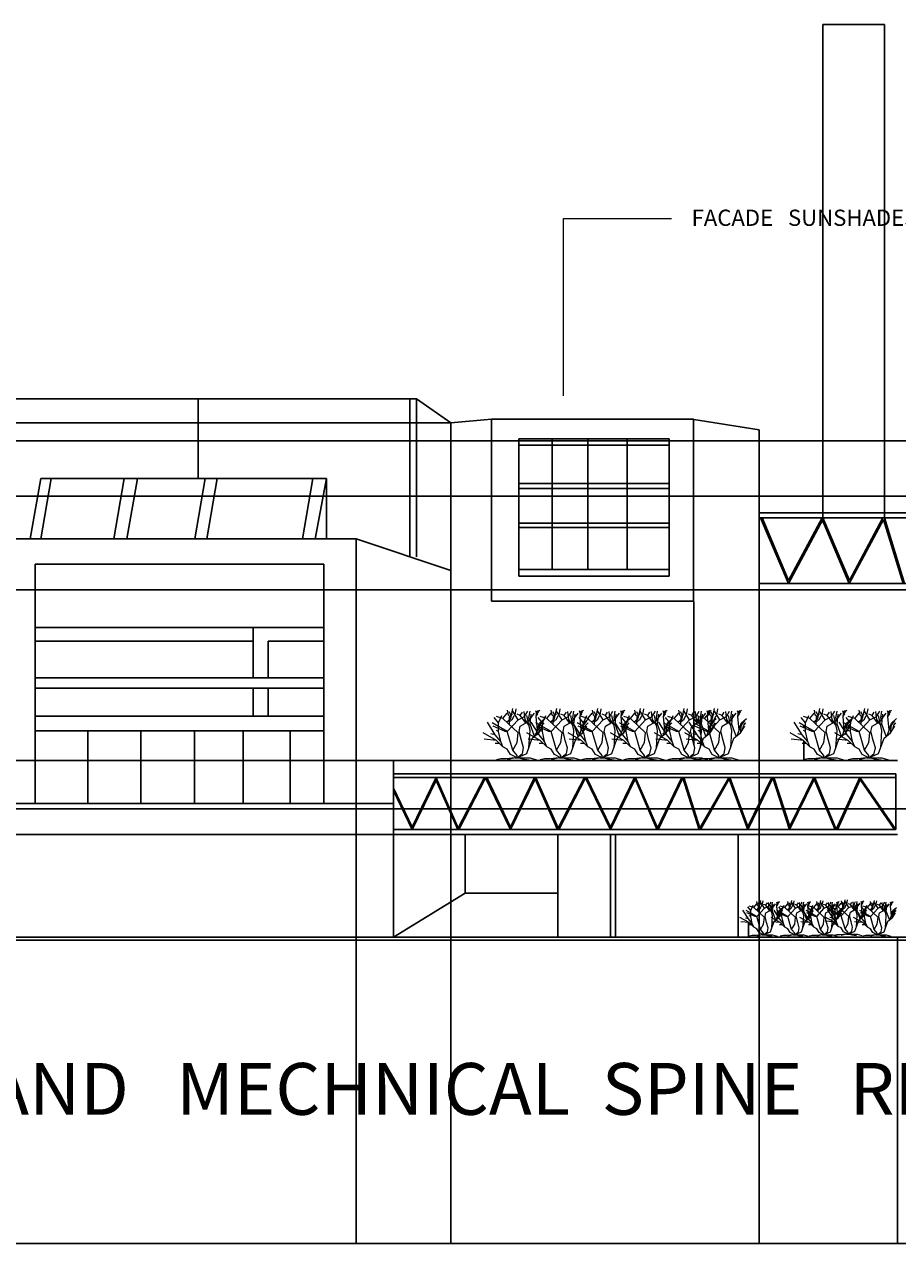
# Model space of a CAD drawing. Units: inches. Extents: x -32109 to 33221, y -19197 to 7608.
# Tile 2 of 25: x -20585 to -12087, y -19197 to -7335. Entities that reach past the tile are written whole.
import ezdxf

# ---------------------------------------------------------------- set-up
doc = ezdxf.new("R2010")
doc.units = ezdxf.units.IN
doc.header["$MEASUREMENT"] = 0
for name, color, linetype, lineweight in [('A-ANNO-DIMS', 2, 'Continuous', 18), ('A-ANNO-NOTE', 2, 'Continuous', 18), ('A-ANNO-TEXT', 7, 'Continuous', 25), ('A-ELEV', 7, 'Continuous', 25), ('L-PLNT', 3, 'Continuous', 13)]:
    doc.layers.add(name, color=color, linetype=linetype, lineweight=lineweight)
doc.styles.get("Standard").update_dxf_attribs({"font": 'arial.ttf'})
doc.dimstyles.get("Standard").update_dxf_attribs({"dimtxt": 0.18, "dimasz": 0.18, "dimexe": 0.18, "dimexo": 0.0625, "dimgap": 0.09, "dimtad": 0, "dimtih": 1, "dimtoh": 1, "dimdec": 4, "dimzin": 0, "dimdsep": 46, "dimtxsty": 'Standard', "dimcen": 0.09, "dimadec": 0, "dimazin": 0, "dimtfac": 1, "dimtdec": 4, "dimtofl": 0, "dimtmove": 0, "dimatfit": 3, "dimfxl": 1, "dimtolj": 1, "dimtzin": 0, "dimarcsym": 0})

# ---------------------------------------------------------------- blocks, each defined once
blk = doc.blocks.new('*U3')
for p, q in [((-12.47099999999977, 19.77499999999986), (-12.89799999999991, 22.04399999999987)), ((-11.43299999999999, 18.28899999999976), (-10.45699999999988, 22.7489999999998)), ((-8.160000000000082, 17.75999999999999), (-10.55999999999994, 21.59999999999991)), ((-9.480000000000018, 19.77499999999986), (-8.991999999999962, 22.59199999999964)), ((-5.279999999999972, 19.19999999999982), (-3.840000000000145, 21.59999999999991)), ((-3.376999999999952, 18.60199999999963), (-2.887999999999919, 21.57499999999982)), ((-0.5079999999998109, 21.88799999999969), (-0.0809999999999036, 20.55799999999976)), ((0.04099999999994, 20.71399999999994), (1.384000000000241, 22.04399999999987)), ((0.1020000000000891, 21.33999999999992), (0.8350000000000363, 21.88799999999969)), ((-18.23999999999978, 11.03999999999996), (-21.75499999999988, 16.65499999999997)), ((-12.95999999999981, 12.47999999999979), (-19.67999999999983, 16.31999999999993)), ((-16.79999999999995, 16.31999999999993), (-18.7199999999998, 18.7199999999998)), ((-14.87999999999988, 18.24000000000001), (-17.75999999999999, 19.19999999999982)), ((-16.79999999999995, 16.31999999999993), (-15.3599999999999, 19.67999999999983)), ((-16.79999999999995, 12.47999999999979), (-16.79999999999995, 16.31999999999993)), ((-14.87999999999988, 18.24000000000001), (-12.95999999999981, 20.63999999999987)), ((-8.160000000000082, 12), (-14.87999999999988, 18.24000000000001)), ((-13.32499999999982, 16.72399999999993), (-11.43299999999999, 18.28899999999976)), ((-12.95999999999981, 12.47999999999979), (-8.160000000000082, 17.75999999999999)), ((-11.67699999999991, 19.07099999999991), (-12.47099999999977, 19.77499999999986)), ((-11.27999999999997, 19.61899999999991), (-12.10400000000004, 21.18399999999974)), ((-12.04299999999989, 15.6279999999997), (-11.92099999999982, 18.83600000000001)), ((-11.98199999999997, 16.80199999999968), (-10.57899999999995, 18.05399999999986)), ((-11.92099999999982, 18.83600000000001), (-10.6400000000001, 20.40100000000007)), ((-10.57899999999995, 18.05399999999986), (-9.845999999999776, 19.69699999999966)), ((-7.200000000000045, 19.67999999999983), (-8.6400000000001, 20.15999999999985)), ((-8.160000000000082, 17.75999999999999), (-5.279999999999972, 19.19999999999982)), ((-7.200000000000045, 19.67999999999983), (-6.240000000000009, 21.11999999999989)), ((-4.799999999999954, 16.31999999999993), (-7.200000000000045, 19.67999999999983)), ((-7.200000000000045, 14.87999999999988), (-3.840000000000145, 16.79999999999995)), ((-5.085999999999785, 17.74099999999998), (-5.512999999999919, 21.33999999999992)), ((-3.376999999999952, 15.31499999999982), (-5.085999999999785, 17.81899999999973)), ((-2.880000000000109, 12.95999999999981), (-4.319999999999936, 19.67999999999983)), ((-3.840000000000145, 16.79999999999995), (-0.9600000000000363, 20.63999999999987)), ((-2.765999999999849, 16.80199999999968), (-3.376999999999952, 18.60199999999963)), ((-2.880000000000109, 15.83999999999992), (-2.40000000000009, 20.15999999999985)), ((-0.2029999999999745, 19.14899999999988), (0.1020000000000891, 21.33999999999992)), ((0.3460000000000036, 13.20299999999974), (-0.2029999999999745, 19.14899999999988)), ((-0.1419999999998254, 19.38399999999979), (0.5899999999999181, 20.40100000000007)), ((-0.0199999999999818, 20.00999999999999), (0.895999999999958, 21.10499999999979)), ((0.3460000000000036, 13.20299999999974), (1.323000000000092, 16.2539999999999)), ((1.323000000000092, 16.2539999999999), (3.642000000000052, 18.28899999999976)), ((1.440000000000054, 15.3599999999999), (2.879999999999881, 17.27999999999997)), ((2.399999999999863, 15.3599999999999), (3.359999999999899, 16.31999999999993)), ((-17.75999999999999, 8.639999999999873), (-23.66300000000001, 11.96100000000001)), ((-18.23999999999978, 11.03999999999996), (-20.15999999999985, 11.51999999999998)), ((-13.91999999999984, 12.47999999999979), (-19.19999999999982, 14.87999999999988)), ((-15.83999999999992, 8.159999999999854), (-18.23999999999978, 11.03999999999996)), ((-16.79999999999995, 12.47999999999979), (-17.75999999999999, 12.95999999999981)), ((-15.83999999999992, 8.159999999999854), (-16.79999999999995, 12.47999999999979)), ((-12.95999999999981, 12.47999999999979), (-13.91999999999984, 12.47999999999979)), ((-10.55999999999994, 4.319999999999936), (-12.95999999999981, 12.47999999999979)), ((-8.6400000000001, 7.679999999999836), (-8.160000000000082, 12)), ((-7.680000000000063, 12.47999999999979), (-7.200000000000045, 14.87999999999988)), ((-6.720000000000027, 8.639999999999873), (-7.680000000000063, 12.47999999999979)), ((-3.360000000000127, 5.279999999999972), (-2.880000000000109, 12.95999999999981)), ((-0.9600000000000363, 10.55999999999994), (-2.880000000000109, 15.83999999999992)), ((-1.920000000000072, 9.599999999999909), (0.9600000000000363, 12)), ((-0.4800000000000182, 10.79999999999995), (0.3460000000000036, 13.20299999999974)), ((0.9600000000000363, 12), (1.440000000000054, 15.3599999999999)), ((0.9600000000000363, 12), (2.879999999999881, 14.87999999999988)), ((1.920000000000072, 13.43999999999982), (2.399999999999863, 15.3599999999999)), ((-17.75999999999999, 8.639999999999873), (-23.12799999999993, 9.221999999999753)), ((-16.31999999999993, 7.199999999999818), (-18.23999999999978, 7.199999999999818)), ((-14.87999999999988, 5.75999999999999), (-17.75999999999999, 8.639999999999873)), ((-14.87999999999988, 5.75999999999999), (-15.83999999999992, 8.159999999999854)), ((-12.95999999999981, 4.799999999999954), (-14.87999999999988, 5.75999999999999)), ((-10.55999999999994, 4.319999999999936), (-8.6400000000001, 7.679999999999836)), ((-5.75999999999999, 5.279999999999972), (-6.720000000000027, 8.639999999999873)), ((-4.319999999999936, 2.879999999999881), (-1.920000000000072, 9.599999999999909)), ((-15.83999999999992, 0.4799999999997909), (-17.75999999999999, 0)), ((-13.43999999999982, 0.4799999999997909), (-15.83999999999992, 0.4799999999997909)), ((-9.600000000000136, 0.959999999999809), (-13.43999999999982, 0.4799999999997909)), ((-11.51999999999998, 2.399999999999863), (-12.95999999999981, 4.799999999999954)), ((-9.600000000000136, 0.959999999999809), (-12.95999999999981, 0)), ((-8.6400000000001, 0.959999999999809), (-11.51999999999998, 2.399999999999863)), ((-8.6400000000001, 1.919999999999845), (-10.55999999999994, 4.319999999999936)), ((-9.600000000000136, 0.959999999999809), (-7.680000000000063, 0.959999999999809)), ((-8.6400000000001, 0.959999999999809), (-4.319999999999936, 2.879999999999881)), ((-8.6400000000001, 0.959999999999809), (-6.240000000000009, 2.879999999999881)), ((-8.6400000000001, 0.959999999999809), (-8.6400000000001, 1.919999999999845)), ((-8.6400000000001, 0.959999999999809), (-2.880000000000109, 0.959999999999809)), ((-7.680000000000063, 0.959999999999809), (-6.240000000000009, 0.4799999999997909)), ((-6.240000000000009, 2.879999999999881), (-5.75999999999999, 5.279999999999972)), ((-6.240000000000009, 0.4799999999997909), (-3.360000000000127, 0)), ((-2.880000000000109, 0.959999999999809), (0, 0))]:
    blk.add_line(p, q)
blk = doc.blocks.new('*D13')
at = {"layer": 'A-ANNO-DIMS', "color": 0, "lineweight": -2, "transparency": 16777216}
for p, q in [((-21916.328365, -16214.873241), (-21916.328365, -19197.348741)), ((5067.151383999999, -16244.175331), (5067.151383999999, -19197.348741)), ((-21916.148365, -19197.168741), (-8425.018722423602, -19197.168741)), ((5066.971383999999, -19197.168741), (-8424.158258576399, -19197.168741))]:
    blk.add_line(p, q, dxfattribs=at)
at = {"layer": 'A-ANNO-DIMS', "color": 0, "transparency": 16777216}
for points in [[(-21916.148365, -19197.138741), (-21916.148365, -19197.198741), (-21916.328365, -19197.168741)], [(5066.971383999999, -19197.138741), (5066.971383999999, -19197.198741), (5067.151383999999, -19197.168741)]]:
    blk.add_solid(points, dxfattribs=at)
at = {"layer": 'Defpoints', "color": 0, "transparency": 16777216}
for p in [(-21916.328365, -16214.810741), (5067.151383999999, -16244.112831), (5067.151383999999, -19197.168741)]:
    blk.add_point(p, dxfattribs=at)
at = {"layer": 'A-ANNO-DIMS', "color": 0, "transparency": 16777216, "insert": (-8424.5884905, -19197.168741), "char_height": 0.18, "attachment_point": 5}
blk.add_mtext('\\A1;26983', dxfattribs=at)
blk = doc.blocks.new('*D14')
at = {"layer": 'A-ANNO-DIMS', "color": 0, "lineweight": -2, "transparency": 16777216}
for p, q in [((-18893.90707200001, -10978.730223), (-32108.36667400003, -10978.73022300001)), ((-32108.18667400003, -10978.91022300001), (-32108.18667400003, -13611.23962386222)), ((-32108.18667400003, -16243.93283100001), (-32108.18667400003, -13611.6034301378)), ((5067.088884000002, -16244.11283100001), (-32108.36667400003, -16244.11283100001))]:
    blk.add_line(p, q, dxfattribs=at)
at = {"layer": 'A-ANNO-DIMS', "color": 0, "transparency": 16777216}
for points in [[(-32108.21667400003, -10978.91022300001), (-32108.15667400003, -10978.91022300001), (-32108.18667400003, -10978.73022300001)], [(-32108.21667400003, -16243.93283100001), (-32108.15667400003, -16243.93283100001), (-32108.18667400003, -16244.11283100001)]]:
    blk.add_solid(points, dxfattribs=at)
at = {"layer": 'Defpoints', "color": 0, "transparency": 16777216}
for p in [(-18893.84457200001, -10978.730223), (-32108.18667400003, -16244.11283100001), (5067.151384000002, -16244.11283100001)]:
    blk.add_point(p, dxfattribs=at)
at = {"layer": 'A-ANNO-DIMS', "color": 0, "transparency": 16777216, "insert": (-32108.18667400002, -13611.421527), "char_height": 0.18, "attachment_point": 5}
blk.add_mtext('\\A1;5265', dxfattribs=at)
blk = doc.blocks.new('*D23')
at = {"layer": 'A-ANNO-DIMS', "color": 0, "lineweight": -2, "transparency": 16777216}
for p, q in [((-4093.737957000001, -14968.07898000001), (-32108.36667400003, -14968.07898000001)), ((-32108.18667400003, -14968.25898000001), (-32108.18667400003, -15591.26295736222)), ((-32108.18667400003, -16214.63074100001), (-32108.18667400003, -15591.6267636378)), ((-4279.014689000002, -16214.810741), (-32108.36667400003, -16214.81074100001))]:
    blk.add_line(p, q, dxfattribs=at)
at = {"layer": 'A-ANNO-DIMS', "color": 0, "transparency": 16777216}
for points in [[(-32108.21667400003, -14968.25898000001), (-32108.15667400003, -14968.25898000001), (-32108.18667400003, -14968.07898000001)], [(-32108.21667400003, -16214.63074100001), (-32108.15667400003, -16214.63074100001), (-32108.18667400003, -16214.81074100001)]]:
    blk.add_solid(points, dxfattribs=at)
at = {"layer": 'Defpoints', "color": 0, "transparency": 16777216}
for p in [(-32108.18667400003, -14968.07898000001), (-4093.675457000002, -14968.07898000001), (-4278.952189000001, -16214.810741)]:
    blk.add_point(p, dxfattribs=at)
at = {"layer": 'A-ANNO-DIMS', "color": 0, "transparency": 16777216, "insert": (-32108.18667400002, -15591.4448605), "char_height": 0.18, "attachment_point": 5}
blk.add_mtext('\\A1;1246.7', dxfattribs=at)
blk = doc.blocks.new('*D79')
at = {"layer": 'A-ANNO-DIMS', "color": 0, "lineweight": -2, "transparency": 16777216}
for p, q in [((-20682.344651, -12340.2456), (-20682.344651, -19197.348741)), ((-17355.072806, -12340.2456), (-17355.072806, -19197.348741)), ((-20682.164651, -19197.168741), (-19019.06743927763, -19197.168741)), ((-17355.252806, -19197.168741), (-19018.35001772237, -19197.168741))]:
    blk.add_line(p, q, dxfattribs=at)
at = {"layer": 'A-ANNO-DIMS', "color": 0, "transparency": 16777216}
for points in [[(-20682.164651, -19197.138741), (-20682.164651, -19197.198741), (-20682.344651, -19197.168741)], [(-17355.252806, -19197.138741), (-17355.252806, -19197.198741), (-17355.072806, -19197.168741)]]:
    blk.add_solid(points, dxfattribs=at)
at = {"layer": 'Defpoints', "color": 0, "transparency": 16777216}
for p in [(-20682.344651, -12340.1831), (-17355.072806, -12340.1831), (-17355.072806, -19197.168741)]:
    blk.add_point(p, dxfattribs=at)
at = {"layer": 'A-ANNO-DIMS', "color": 0, "transparency": 16777216, "insert": (-19018.7087285, -19197.168741), "char_height": 0.18, "attachment_point": 5}
blk.add_mtext('\\A1;3327', dxfattribs=at)
blk = doc.blocks.new('*D80')
at = {"layer": 'A-ANNO-DIMS', "color": 0, "lineweight": -2, "transparency": 16777216}
for p, q in [((-16435.771195, -11210.808758), (-16435.771195, -19197.348741)), ((-17355.072806, -12340.2456), (-17355.072806, -19197.348741)), ((-17354.892806, -19197.168741), (-16895.81570445634, -19197.168741)), ((-16435.951195, -19197.168741), (-16895.02829654366, -19197.168741))]:
    blk.add_line(p, q, dxfattribs=at)
at = {"layer": 'A-ANNO-DIMS', "color": 0, "transparency": 16777216}
for points in [[(-17354.892806, -19197.138741), (-17354.892806, -19197.198741), (-17355.072806, -19197.168741)], [(-16435.951195, -19197.138741), (-16435.951195, -19197.198741), (-16435.771195, -19197.168741)]]:
    blk.add_solid(points, dxfattribs=at)
at = {"layer": 'Defpoints', "color": 0, "transparency": 16777216}
for p in [(-16435.771195, -11210.746258), (-17355.072806, -12340.1831), (-16435.771195, -19197.168741)]:
    blk.add_point(p, dxfattribs=at)
at = {"layer": 'A-ANNO-DIMS', "color": 0, "transparency": 16777216, "insert": (-16895.4220005, -19197.168741), "char_height": 0.18, "attachment_point": 5}
blk.add_mtext('\\A1;919.3', dxfattribs=at)
blk = doc.blocks.new('*D81')
at = {"layer": 'A-ANNO-DIMS', "color": 0, "lineweight": -2, "transparency": 16777216}
for p, q in [((-16435.771195, -11210.808758), (-16435.771195, -19197.348741)), ((-13434.382943, -11279.930606), (-13434.382943, -19197.348741)), ((-16435.591195, -19197.168741), (-14935.54026818144, -19197.168741)), ((-13434.562943, -19197.168741), (-14934.61386981855, -19197.168741))]:
    blk.add_line(p, q, dxfattribs=at)
at = {"layer": 'A-ANNO-DIMS', "color": 0, "transparency": 16777216}
for points in [[(-16435.591195, -19197.138741), (-16435.591195, -19197.198741), (-16435.771195, -19197.168741)], [(-13434.562943, -19197.138741), (-13434.562943, -19197.198741), (-13434.382943, -19197.168741)]]:
    blk.add_solid(points, dxfattribs=at)
at = {"layer": 'Defpoints', "color": 0, "transparency": 16777216}
for p in [(-16435.771195, -11210.746258), (-13434.382943, -11279.868106), (-13434.382943, -19197.168741)]:
    blk.add_point(p, dxfattribs=at)
at = {"layer": 'A-ANNO-DIMS', "color": 0, "transparency": 16777216, "insert": (-14935.077069, -19197.168741), "char_height": 0.18, "attachment_point": 5}
blk.add_mtext('\\A1;3001.4', dxfattribs=at)
blk = doc.blocks.new('*D82')
at = {"layer": 'A-ANNO-DIMS', "color": 0, "lineweight": -2, "transparency": 16777216}
for p, q in [((-13434.382943, -11279.930606), (-13434.382943, -19197.348741)), ((-12087.22567, -16214.873241), (-12087.22567, -19197.348741)), ((-13434.202943, -19197.168741), (-12761.25854251637, -19197.168741)), ((-12087.40567, -19197.168741), (-12760.35007048363, -19197.168741))]:
    blk.add_line(p, q, dxfattribs=at)
at = {"layer": 'A-ANNO-DIMS', "color": 0, "transparency": 16777216}
for points in [[(-13434.202943, -19197.138741), (-13434.202943, -19197.198741), (-13434.382943, -19197.168741)], [(-12087.40567, -19197.138741), (-12087.40567, -19197.198741), (-12087.22567, -19197.168741)]]:
    blk.add_solid(points, dxfattribs=at)
at = {"layer": 'Defpoints', "color": 0, "transparency": 16777216}
for p in [(-13434.382943, -11279.868106), (-12087.22567, -16214.810741), (-12087.22567, -19197.168741)]:
    blk.add_point(p, dxfattribs=at)
at = {"layer": 'A-ANNO-DIMS', "color": 0, "transparency": 16777216, "insert": (-12760.8043065, -19197.168741), "char_height": 0.18, "attachment_point": 5}
blk.add_mtext('\\A1;1347.2', dxfattribs=at)
blk = doc.blocks.new('*D83')
at = {"layer": 'A-ANNO-DIMS', "color": 0, "lineweight": -2, "transparency": 16777216}
for p, q in [((-12087.22567, -16214.873241), (-12087.22567, -19197.348741)), ((-8664.142997, -16214.873241), (-8664.142997, -19197.348741)), ((-12087.04567, -19197.168741), (-10376.04304427762, -19197.168741)), ((-8664.322997000001, -19197.168741), (-10375.32562272237, -19197.168741))]:
    blk.add_line(p, q, dxfattribs=at)
at = {"layer": 'A-ANNO-DIMS', "color": 0, "transparency": 16777216}
for points in [[(-12087.04567, -19197.138741), (-12087.04567, -19197.198741), (-12087.22567, -19197.168741)], [(-8664.322997000001, -19197.138741), (-8664.322997000001, -19197.198741), (-8664.142997, -19197.168741)]]:
    blk.add_solid(points, dxfattribs=at)
at = {"layer": 'Defpoints', "color": 0, "transparency": 16777216}
for p in [(-12087.22567, -16214.810741), (-8664.142997, -16214.810741), (-8664.142997, -19197.168741)]:
    blk.add_point(p, dxfattribs=at)
at = {"layer": 'A-ANNO-DIMS', "color": 0, "transparency": 16777216, "insert": (-10375.6843335, -19197.168741), "char_height": 0.18, "attachment_point": 5}
blk.add_mtext('\\A1;3423', dxfattribs=at)
blk = doc.blocks.new('*D86')
at = {"layer": 'A-ANNO-DIMS', "color": 0, "lineweight": -2, "transparency": 16777216}
for p, q in [((-18893.90707200001, -10978.730223), (-32108.36667400003, -10978.73022300001)), ((-32108.18667400003, -10978.91022300001), (-32108.18667400003, -11659.27469697068)), ((-32108.18667400003, -12340.00310000001), (-32108.18667400003, -11659.63862602934)), ((-17355.13530600001, -12340.18310000001), (-32108.36667400003, -12340.18310000001))]:
    blk.add_line(p, q, dxfattribs=at)
at = {"layer": 'A-ANNO-DIMS', "color": 0, "transparency": 16777216}
for points in [[(-32108.21667400003, -10978.91022300001), (-32108.15667400003, -10978.91022300001), (-32108.18667400003, -10978.73022300001)], [(-32108.21667400003, -12340.00310000001), (-32108.15667400003, -12340.00310000001), (-32108.18667400003, -12340.18310000001)]]:
    blk.add_solid(points, dxfattribs=at)
at = {"layer": 'Defpoints', "color": 0, "transparency": 16777216}
for p in [(-18893.84457200001, -10978.730223), (-32108.18667400003, -12340.18310000001), (-17355.07280600001, -12340.18310000001)]:
    blk.add_point(p, dxfattribs=at)
at = {"layer": 'A-ANNO-DIMS', "color": 0, "transparency": 16777216, "insert": (-32108.18667400002, -11659.4566615), "char_height": 0.18, "attachment_point": 5}
blk.add_mtext('\\A1;1361.5', dxfattribs=at)
blk = doc.blocks.new('*D87')
at = {"layer": 'A-ANNO-DIMS', "color": 0, "lineweight": -2, "transparency": 16777216}
for p, q in [((-16435.83369500001, -11210.746258), (-32108.36667400003, -11210.746258)), ((-32108.18667400003, -11210.926258), (-32108.18667400003, -13712.59659636222)), ((-32108.18667400003, -16214.63074100001), (-32108.18667400003, -13712.96040263779)), ((-16994.015761, -16214.810741), (-32108.36667400003, -16214.81074100001))]:
    blk.add_line(p, q, dxfattribs=at)
at = {"layer": 'A-ANNO-DIMS', "color": 0, "transparency": 16777216}
for points in [[(-32108.21667400003, -11210.926258), (-32108.15667400003, -11210.926258), (-32108.18667400003, -11210.746258)], [(-32108.21667400003, -16214.63074100001), (-32108.15667400003, -16214.63074100001), (-32108.18667400003, -16214.81074100001)]]:
    blk.add_solid(points, dxfattribs=at)
at = {"layer": 'Defpoints', "color": 0, "transparency": 16777216}
for p in [(-16435.77119500001, -11210.746258), (-32108.18667400003, -16214.81074100001), (-16993.95326100001, -16214.810741)]:
    blk.add_point(p, dxfattribs=at)
at = {"layer": 'A-ANNO-DIMS', "color": 0, "transparency": 16777216, "insert": (-32108.18667400002, -13712.77849949999), "char_height": 0.18, "attachment_point": 5}
blk.add_mtext('\\A1;5004', dxfattribs=at)
blk = doc.blocks.new('*D88')
at = {"layer": 'A-ANNO-DIMS', "color": 0, "lineweight": -2, "transparency": 16777216}
for p, q in [((-6450.017839000004, -11923.964476), (-32108.36667400003, -11923.964476)), ((-32108.18667400003, -11924.144476), (-32108.18667400003, -12380.67353997068)), ((-32108.18667400003, -12837.56653300001), (-32108.18667400003, -12381.03746902934)), ((-6450.017839000004, -12837.746533), (-32108.36667400003, -12837.74653300001))]:
    blk.add_line(p, q, dxfattribs=at)
at = {"layer": 'A-ANNO-DIMS', "color": 0, "transparency": 16777216}
for points in [[(-32108.21667400003, -11924.144476), (-32108.15667400003, -11924.144476), (-32108.18667400003, -11923.964476)], [(-32108.21667400003, -12837.56653300001), (-32108.15667400003, -12837.56653300001), (-32108.18667400003, -12837.74653300001)]]:
    blk.add_solid(points, dxfattribs=at)
at = {"layer": 'Defpoints', "color": 0, "transparency": 16777216}
for p in [(-6449.955339000005, -11923.964476), (-32108.18667400003, -12837.74653300001), (-6449.955339000005, -12837.746533)]:
    blk.add_point(p, dxfattribs=at)
at = {"layer": 'A-ANNO-DIMS', "color": 0, "transparency": 16777216, "insert": (-32108.18667400002, -12380.8555045), "char_height": 0.18, "attachment_point": 5}
blk.add_mtext('\\A1;913.8', dxfattribs=at)
blk = doc.blocks.new('*D89')
at = {"layer": 'A-ANNO-DIMS', "color": 0, "lineweight": -2, "transparency": 16777216}
for p, q in [((-13434.44544300001, -12837.746533), (-32108.36667400003, -12837.74653300001)), ((-32108.18667400003, -12837.92653300001), (-32108.18667400003, -14526.09667247068)), ((-32108.18667400003, -16214.63074100001), (-32108.18667400003, -14526.46060152934)), ((-12087.28817, -16214.810741), (-32108.36667400003, -16214.81074100001))]:
    blk.add_line(p, q, dxfattribs=at)
at = {"layer": 'A-ANNO-DIMS', "color": 0, "transparency": 16777216}
for points in [[(-32108.21667400003, -12837.92653300001), (-32108.15667400003, -12837.92653300001), (-32108.18667400003, -12837.74653300001)], [(-32108.21667400003, -16214.63074100001), (-32108.15667400003, -16214.63074100001), (-32108.18667400003, -16214.81074100001)]]:
    blk.add_solid(points, dxfattribs=at)
at = {"layer": 'Defpoints', "color": 0, "transparency": 16777216}
for p in [(-13434.38294300001, -12837.746533), (-32108.18667400003, -16214.81074100001), (-12087.22567, -16214.810741)]:
    blk.add_point(p, dxfattribs=at)
at = {"layer": 'A-ANNO-DIMS', "color": 0, "transparency": 16777216, "insert": (-32108.18667400002, -14526.278637), "char_height": 0.18, "attachment_point": 5}
blk.add_mtext('\\A1;3377', dxfattribs=at)
blk = doc.blocks.new('*D90')
at = {"layer": 'A-ANNO-DIMS', "color": 0, "lineweight": -2, "transparency": 16777216}
for p, q in [((-16994.015761, -14496.89128100001), (-32108.36667400003, -14496.89128100001)), ((-32108.18667400003, -14497.07128100001), (-32108.18667400003, -14856.96167986222)), ((-32108.18667400003, -15217.21588500001), (-32108.18667400003, -14857.32548613779)), ((-16994.015761, -15217.395885), (-32108.36667400003, -15217.39588500001))]:
    blk.add_line(p, q, dxfattribs=at)
at = {"layer": 'A-ANNO-DIMS', "color": 0, "transparency": 16777216}
for points in [[(-32108.21667400003, -14497.07128100001), (-32108.15667400003, -14497.07128100001), (-32108.18667400003, -14496.89128100001)], [(-32108.21667400003, -15217.21588500001), (-32108.15667400003, -15217.21588500001), (-32108.18667400003, -15217.39588500001)]]:
    blk.add_solid(points, dxfattribs=at)
at = {"layer": 'Defpoints', "color": 0, "transparency": 16777216}
for p in [(-16993.95326100001, -14496.89128100001), (-32108.18667400003, -15217.39588500001), (-16993.95326100001, -15217.395885)]:
    blk.add_point(p, dxfattribs=at)
at = {"layer": 'A-ANNO-DIMS', "color": 0, "transparency": 16777216, "insert": (-32108.18667400002, -14857.14358299999), "char_height": 0.18, "attachment_point": 5}
blk.add_mtext('\\A1;720.5', dxfattribs=at)
blk = doc.blocks.new('*D91')
at = {"layer": 'A-ANNO-DIMS', "color": 0, "lineweight": -2, "transparency": 16777216}
for p, q in [((-16994.015761, -15217.395885), (-32108.36667400003, -15217.39588500001)), ((-32108.18667400003, -15217.57588500001), (-32108.18667400003, -15715.92140986222)), ((-32108.18667400003, -16214.63074100001), (-32108.18667400003, -15716.2852161378)), ((-16994.015761, -16214.810741), (-32108.36667400003, -16214.81074100001))]:
    blk.add_line(p, q, dxfattribs=at)
at = {"layer": 'A-ANNO-DIMS', "color": 0, "transparency": 16777216}
for points in [[(-32108.21667400003, -15217.57588500001), (-32108.15667400003, -15217.57588500001), (-32108.18667400003, -15217.39588500001)], [(-32108.21667400003, -16214.63074100001), (-32108.15667400003, -16214.63074100001), (-32108.18667400003, -16214.81074100001)]]:
    blk.add_solid(points, dxfattribs=at)
at = {"layer": 'Defpoints', "color": 0, "transparency": 16777216}
for p in [(-16993.95326100001, -15217.395885), (-32108.18667400003, -16214.81074100001), (-16993.95326100001, -16214.810741)]:
    blk.add_point(p, dxfattribs=at)
at = {"layer": 'A-ANNO-DIMS', "color": 0, "transparency": 16777216, "insert": (-32108.18667400002, -15716.10331299999), "char_height": 0.18, "attachment_point": 5}
blk.add_mtext('\\A1;997.4', dxfattribs=at)
blk = doc.blocks.new('*D93')
at = {"layer": 'A-ANNO-DIMS', "color": 0, "lineweight": -2, "transparency": 16777216}
for p, q in [((-12813.954106, -12135.102), (-12813.954106, -7334.980009999999)), ((-12813.774106, -7335.16001), (-12515.24987308322, -7335.16001)), ((-12215.940074, -7335.16001), (-12514.46430691678, -7335.16001)), ((-12215.760074, -12135.984869), (-12215.760074, -7334.980009999999))]:
    blk.add_line(p, q, dxfattribs=at)
at = {"layer": 'A-ANNO-DIMS', "color": 0, "transparency": 16777216}
for points in [[(-12813.774106, -7335.13001), (-12813.774106, -7335.190009999999), (-12813.954106, -7335.16001)], [(-12215.940074, -7335.13001), (-12215.940074, -7335.190009999999), (-12215.760074, -7335.16001)]]:
    blk.add_solid(points, dxfattribs=at)
at = {"layer": 'Defpoints', "color": 0, "transparency": 16777216}
for p in [(-12215.760074, -7335.16001), (-12813.954106, -12135.1645), (-12215.760074, -12136.047369)]:
    blk.add_point(p, dxfattribs=at)
at = {"layer": 'A-ANNO-DIMS', "color": 0, "transparency": 16777216, "insert": (-12514.85709, -7335.16001), "char_height": 0.18, "attachment_point": 5}
blk.add_mtext('\\A1;598.2', dxfattribs=at)
blk = doc.blocks.new('*D159')
at = {"layer": 'A-ANNO-DIMS', "color": 0, "lineweight": -2, "transparency": 16777216}
for p, q in [((-6094.734242000003, -11386.25619), (-32108.36667400003, -11386.25619000001)), ((-32108.18667400003, -11386.43619000001), (-32108.18667400003, -13800.35156236222)), ((-32108.18667400003, -16214.63074100001), (-32108.18667400003, -13800.7153686378)), ((-6952.836375000003, -16214.810741), (-32108.36667400003, -16214.81074100001))]:
    blk.add_line(p, q, dxfattribs=at)
at = {"layer": 'A-ANNO-DIMS', "color": 0, "transparency": 16777216}
for points in [[(-32108.21667400003, -11386.43619000001), (-32108.15667400003, -11386.43619000001), (-32108.18667400003, -11386.25619000001)], [(-32108.21667400003, -16214.63074100001), (-32108.15667400003, -16214.63074100001), (-32108.18667400003, -16214.81074100001)]]:
    blk.add_solid(points, dxfattribs=at)
at = {"layer": 'Defpoints', "color": 0, "transparency": 16777216}
for p in [(-6094.671742000002, -11386.25619), (-32108.18667400003, -16214.81074100001), (-6952.773875000004, -16214.810741)]:
    blk.add_point(p, dxfattribs=at)
at = {"layer": 'A-ANNO-DIMS', "color": 0, "transparency": 16777216, "insert": (-32108.18667400002, -13800.5334655), "char_height": 0.18, "attachment_point": 5}
blk.add_mtext('\\A1;4828.6', dxfattribs=at)

msp = doc.modelspace()

# ---------------------------------------------------------------- linework, layer by layer
at = {"layer": 'A-ANNO-NOTE'}
for p, q in [((-15340.20223612337, -10950.51521976139), (-15340.20223612337, -9225.160009906325)), ((-15340.20223612337, -9225.160009906325), (-14287.5535247844, -9225.160009906325))]:
    msp.add_line(p, q, dxfattribs=at)
at = {"layer": 'A-ELEV'}
for p, q in [((-16769.4226129395, -10978.73022341639), (-18893.84457171501, -10978.73022341639)), ((-18893.84457171501, -10978.73022341639), (-18893.84457171501, -11753.08186998484)), ((-16832.48196013175, -12514.52263236995), (-16832.48196013174, -10978.73022341639)), ((-16769.4226129395, -12514.52263236995), (-16769.4226129395, -10978.73022341639)), ((-16769.4226129395, -10978.73022341639), (-16435.77119529921, -11210.74625835801)), ((-16039.7342330258, -11175.08856378732), (-16435.77119529921, -11210.74625835801)), ((-16435.77119529921, -11210.74625835801), (-16435.77119529921, -12448.88513076392)), ((-16039.73423302581, -11175.08856378732), (-14074.15321761477, -11175.08856378732)), ((-16039.7342330258, -11646.16850562423), (-16039.7342330258, -11175.08856378732)), ((-14074.15321761477, -11175.08856378732), (-14074.15321761477, -12946.27528221659)), ((-13434.38294252073, -11279.86810558472), (-14071.59279220595, -11179.17208158662)), ((-15772.70986409412, -12703.71369814485), (-15772.70986409412, -11367.54375505061)), ((-15772.70986409412, -11367.54375505061), (-14309.90954077573, -11367.54375505061)), ((-15449.03562252067, -12639.40078018609), (-15449.03562252067, -11367.54375505061)), ((-15102.10281071182, -12639.40078018609), (-15102.10281071182, -11367.54375505061)), ((-14717.80837918442, -12639.40078018609), (-14717.80837918442, -11367.54375505061)), ((-14309.90954077573, -11367.54375505061), (-14309.90954077573, -12703.71369814485)), ((-13434.38294252073, -14496.89128132054), (-13434.38294252073, -11279.86810558472)), ((-15772.70986409412, -11430.01415629164), (-14309.90954077573, -11430.01415629164)), ((-16039.7342330258, -12183.95817617406), (-16039.7342330258, -11646.16850562423)), ((-20527.96552109694, -12340.18310009528), (-20426.04896038951, -11753.08186998484)), ((-20426.40863988602, -12340.18310009528), (-20324.49207917859, -11753.08186998484)), ((-20426.04896038951, -11753.08186998484), (-17644.28538792832, -11753.08186998484)), ((-19715.1139285969, -12340.18310009528), (-19613.19736788947, -11753.08186998484)), ((-19586.73392241359, -12340.18310009528), (-19484.81736170616, -11753.08186998484)), ((-18927.48504543547, -12340.18310009528), (-18825.56848472804, -11753.08186998484)), ((-18809.51415918945, -12340.18310009528), (-18707.59759848202, -11753.08186998484)), ((-17879.62652146987, -12340.18310009528), (-17777.70996076244, -11753.08186998484)), ((-17644.28538792832, -11753.08186998484), (-17755.14429501962, -12340.18310009528)), ((-17644.28538792832, -11753.08186998484), (-17644.28538792831, -12340.18310009528)), ((-15772.70986409412, -11802.32034552261), (-14309.90954077573, -11802.32034552261)), ((-15772.70986409412, -11849.9533244479), (-14309.90954077573, -11849.9533244479)), ((-6449.955339184301, -11923.96447596985), (-13434.38294252073, -11923.96447596985)), ((-13434.38294252073, -12088.72486351584), (-6449.955339184301, -12088.72486351584)), ((-16039.7342330258, -12183.95817617406), (-16039.73423302581, -12292.66020684269)), ((-15772.70986409412, -12186.8873610721), (-14309.90954077573, -12186.8873610721)), ((-6449.955339184301, -12135.16449966414), (-13434.38294252073, -12135.16449966414)), ((-13149.46023596293, -12774.36220746369), (-13420.24211770431, -12134.94326833175)), ((-13148.11921329626, -12744.75684322936), (-13406.27009339034, -12135.16449966414)), ((-12816.57529212094, -12151.93909962213), (-13149.46023596293, -12774.36220746369)), ((-12822.09643152984, -12135.16449966414), (-13148.11921329627, -12744.75684322935)), ((-12827.92613029018, -12135.16449966414), (-12827.92613029018, -12134.94326833175)), ((-12557.1442485488, -12774.36220746369), (-12827.92613029018, -12134.94326833175)), ((-12555.80322588213, -12744.75684322936), (-12813.95410597621, -12135.16449966414)), ((-12224.25930470681, -12151.93909962213), (-12557.1442485488, -12774.36220746369)), ((-12229.78044411572, -12135.16449966414), (-12555.80322588214, -12744.75684322935)), ((-12033.80773837084, -12773.91673601398), (-12224.25930470682, -12151.93909962213)), ((-12020.32553277507, -12774.2984277213), (-12215.76007366987, -12136.04736917849)), ((-16039.7342330258, -12292.66020684269), (-16039.7342330258, -12946.27528221659)), ((-15772.70986409412, -12228.56624746265), (-14309.90954077573, -12228.56624746265)), ((-18893.84457171501, -12340.18310009528), (-20682.34465069239, -12340.18310009528)), ((-18893.84457171501, -12340.18310009528), (-17355.07280614063, -12340.18310009528)), ((-17355.07280614063, -12340.18310009528), (-17355.07280614063, -14914.70396449454)), ((-17355.07280614063, -12340.18310009528), (-16435.77119529921, -12646.8677924841)), ((-16435.77119529921, -12340.18310009528), (-16435.77119529921, -12646.8677924841)), ((-20480.4645030599, -14914.70396449454), (-20480.4645030599, -12587.3189270875)), ((-20480.4645030599, -12587.3189270875), (-17669.73347483821, -12587.3189270875)), ((-17669.73347483821, -12587.3189270875), (-20480.4645030599, -12587.3189270875)), ((-17669.73347483821, -12587.3189270875), (-17669.73347483821, -14914.70396449454)), ((-16435.77119529921, -12646.8677924841), (-16435.77119529921, -14496.89128132054)), ((-15772.70986409412, -12639.40078018609), (-14309.90954077573, -12639.40078018609)), ((-14309.90954077573, -12703.71369814485), (-15772.70986409412, -12703.71369814485)), ((-13434.38294252073, -12773.91673601398), (-6449.955339184301, -12773.91673601398)), ((-6449.955339184301, -12837.74653340205), (-13434.38294252073, -12837.74653340205)), ((-14074.15321761477, -12946.27528221659), (-16039.7342330258, -12946.27528221659)), ((-14074.15321761477, -12946.27528221659), (-14255.31722758227, -12946.27528221659)), ((-14071.59279220595, -13488.14847056572), (-14071.59279220595, -12950.35880001589)), ((-17669.73347483821, -13204.32128453172), (-20480.4645030599, -13204.32128453172)), ((-18358.49718674543, -13204.32128453172), (-18358.49718674543, -13691.10200328602)), ((-18358.49718674543, -13336.53337146936), (-20480.4645030599, -13336.53337146936)), ((-17669.73347483821, -13336.53337146936), (-18214.09302493594, -13336.53337146936)), ((-18214.09302493593, -13336.53337146936), (-18214.09302493593, -13691.10200328602)), ((-14071.59279220595, -13488.14847056572), (-14071.59279220594, -14344.74987519862)), ((-17669.73347483821, -13691.10200328602), (-20480.4645030599, -13691.10200328602)), ((-17669.73347483821, -13793.26584787226), (-20480.4645030599, -13793.26584787226)), ((-18358.49718674543, -13793.26584787226), (-18358.49718674543, -14066.58814800302)), ((-18214.09302493593, -13793.26584787226), (-18214.09302493593, -14066.58814800302)), ((-18358.49718674543, -14066.58814800302), (-20480.4645030599, -14066.58814800302)), ((-18358.49718674543, -14066.58814800302), (-18214.09302493593, -14066.58814800302)), ((-17669.73347483821, -14066.58814800302), (-18214.09302493593, -14066.58814800302)), ((-17669.73347483821, -14207.93087468744), (-20480.4645030599, -14207.93087468744)), ((-19966.10757241401, -14914.70396449454), (-19966.10757241401, -14207.93087468744)), ((-19451.28139258801, -14914.70396449454), (-19451.28139258801, -14207.93087468744)), ((-18928.01553163354, -14914.70396449454), (-18928.01553163354, -14207.93087468744)), ((-18455.38822669901, -14914.70396449454), (-18455.38822669901, -14207.93087468744)), ((-17999.64051864595, -14914.70396449454), (-17999.64051864595, -14207.93087468744)), ((-13000.13529992214, -14179.87897816674), (-13000.13529992214, -14158.42745826966)), ((-13000.13529992214, -14496.89128132054), (-13000.13529992214, -14305.16534370231)), ((-12087.69592444187, -14496.89128132054), (-16993.95326078704, -14496.89128132054)), ((-16993.95326078703, -14914.70396449454), (-16993.95326078703, -14496.89128132054)), ((-16993.95326078704, -14626.80258426852), (-12106.11998465589, -14626.80258426852)), ((-12106.11998465589, -14663.41959962224), (-16993.95326078704, -14663.41959962224)), ((-16572.21491409015, -14676.06364930675), (-16811.17299060459, -15167.38737566869)), ((-16577.27054501888, -14663.41959962224), (-16811.14945209219, -15144.30000264881)), ((-16368.60279732297, -15167.06696608635), (-16585.27440689767, -14675.57265962713)), ((-16362.64417428292, -15155.60334164811), (-16579.20831355345, -14664.35281905481)), ((-16107.80286276937, -14663.41959962224), (-16362.64417428292, -15155.60334164811)), ((-16096.89840619271, -14664.2746617505), (-16357.42591591668, -15167.4403528822)), ((-15853.4739862697, -15167.38737566869), (-16096.89840619271, -14664.2746617505)), ((-15853.4504477573, -15144.30000264881), (-16086.11805865397, -14663.41959962224)), ((-15614.51590975527, -14676.06364930675), (-15853.4739862697, -15167.38737566869)), ((-15619.57154068399, -14663.41959962224), (-15853.4504477573, -15144.30000264881)), ((-15396.66270818206, -15167.06696608635), (-15613.33431775676, -14675.57265962713)), ((-15390.70408514202, -15155.60334164811), (-15607.26822441254, -14664.35281905481)), ((-15135.86277362846, -14663.41959962224), (-15390.70408514202, -15155.60334164811)), ((-15124.9583170518, -14664.2746617505), (-15385.48582677577, -15167.4403528822)), ((-14881.5338971288, -15167.38737566869), (-15124.9583170518, -14664.2746617505)), ((-14881.51035861639, -15144.30000264881), (-15114.17796951306, -14663.41959962224)), ((-14642.57582061436, -14676.06364930675), (-14881.5338971288, -15167.38737566869)), ((-14647.63145154308, -14663.41959962224), (-14881.51035861639, -15144.30000264881)), ((-14425.7695026686, -15171.36934092964), (-14642.57582061436, -14676.06364930675)), ((-14416.53853258838, -15167.32874000781), (-14636.78655459714, -14664.16029038302)), ((-14188.20323315877, -14663.41959962224), (-14425.63952522038, -15163.0033270167)), ((-14177.3666678331, -14664.09323778169), (-14416.53853258838, -15167.32874000781)), ((-14018.07612665022, -15167.06696608635), (-14177.3666678331, -14664.09323778169)), ((-14010.75102709925, -15156.82146639105), (-14167.0101833044, -14663.41959962224)), ((-13731.27054126968, -14664.45863202064), (-14010.75102709925, -15156.82146639106)), ((-13726.6967789477, -14676.81348822869), (-14004.97992829729, -15167.06696608635)), ((-13545.14341466165, -15167.23374882259), (-13726.6967789477, -14676.81348822869)), ((-13543.8857755777, -15141.60634555062), (-13720.91029812732, -14663.41959962224)), ((-13300.59550026204, -14664.35543608672), (-13545.14341466165, -15167.23374882259)), ((-13311.34528128967, -14663.41959962224), (-13543.8857755777, -15141.60634555063)), ((-13139.48143436485, -15167.23374882259), (-13300.59550026204, -14664.35543608672)), ((-13137.51489620357, -15140.34549841396), (-13290.31422904408, -14663.41959962224)), ((-12899.40074486054, -14677.83105750947), (-13139.48143436485, -15167.23374882259)), ((-12902.54163801712, -14661.35426767196), (-13137.51489620357, -15140.34549841396)), ((-12695.89294774142, -15167.06696608635), (-12899.40074486054, -14677.83105750947)), ((-12684.90998218706, -15167.23374882259), (-12893.4949734396, -14665.79218660464)), ((-12454.74734804524, -14661.48179358967), (-12684.90998218706, -15167.23374882259)), ((-12452.94439951792, -14681.84704058144), (-12673.76311319126, -15167.06696608635)), ((-12106.11998465589, -15167.06696608635), (-12454.74734804524, -14661.48179358967)), ((-12118.35993681027, -15167.06696608635), (-12452.94439951792, -14681.84704058144)), ((-12106.11998465589, -15167.06696608635), (-12106.11998465589, -14626.80258426852)), ((-16811.14945209219, -15144.30000264881), (-16993.95326078703, -14766.47874570123)), ((-16811.17299060459, -15167.38737566869), (-16993.95326078703, -14789.61476842052)), ((-20682.34465069239, -14914.70396449454), (-16993.95326078703, -14914.70396449454)), ((-16993.95326078703, -14914.70396449454), (-16993.95326078701, -16214.8107410869)), ((-16993.95326078704, -15167.06696608635), (-12106.11998465589, -15167.06696608635)), ((-16357.42591591668, -15167.4403528822), (-16357.59052070861, -15167.06696608635)), ((-15385.48582677577, -15167.4403528822), (-15385.6504315677, -15167.06696608635)), ((-12087.69592444187, -15217.3958847609), (-16993.95326078704, -15217.3958847609)), ((-16295.59376672657, -15789.16679527706), (-16295.59376672657, -15217.3958847609)), ((-15392.8334422986, -15217.39588476091), (-15392.83344229861, -16214.8107410869)), ((-14881.37806411405, -15217.3958847609), (-14881.37806411406, -16214.81074108689)), ((-14832.69023734145, -15217.3958847609), (-14832.69023734146, -16214.81074108689)), ((-13637.34514960736, -15217.3958847609), (-13637.34514960736, -15930.15875459481)), ((-16993.95326078701, -16214.8107410869), (-16295.59376672657, -15789.16679527706)), ((-16295.59376672657, -15789.16679527706), (-15392.83344229861, -15789.16679527706)), ((-13637.34514960736, -15930.15875459481), (-13637.34514960736, -16214.81074108689)), ((-13537.91264792656, -16070.6734389156), (-13537.91264792656, -16214.81074108689)), ((-16993.95326078701, -16214.8107410869), (-24194.61444585808, -16214.8107410869)), ((-16993.95326078701, -16214.8107410869), (-13538.06619730289, -16214.8107410869))]:
    msp.add_line(p, q, dxfattribs=at)

# ---------------------------------------------------------------- block references
at = {"layer": 'L-PLNT'}
for p, xscale, yscale, zscale in [((-15600.58101547453, -14491.04286245773), 22.01107992076033, 22.01107992076033, 22.01107992076033), ((-15173.65553056081, -14491.04286245773), 22.01107992076033, 22.01107992076033, 22.01107992076033), ((-14772.91203827466, -14491.04286245773), 22.01107992076033, 22.01107992076033, 22.01107992076033), ((-14359.61190717853, -14491.04286245773), 22.01107992076033, 22.01107992076033, 22.01107992076033), ((-13932.6866568894, -14491.04286245773), 22.01107992076033, 22.01107992076033, 22.01107992076033), ((-13637.4723780884, -14491.04286245773), 22.01107992076033, 22.01107992076033, 22.01107992076033), ((-12613.51673228938, -14491.04286245773), 22.01107992076033, 22.01107992076033, 22.01107992076033), ((-12177.24715875513, -14491.04286245773), 22.01107992076033, 22.01107992076033, 22.01107992076033), ((-13259.37770991711, -16206.68344137856), 15.30854395898754, 15.30854395898754, 15.30854395898754), ((-12956.81438919035, -16206.68344137856), 15.30854395898754, 15.30854395898754, 15.30854395898754), ((-12675.66515068872, -16206.68344137856), 15.30854395898754, 15.30854395898754, 15.30854395898754), ((-12436.84684903007, -16200.03136298989), 15.30854395898754, 15.30854395898754, 15.30854395898754), ((-12153.05835020771, -16206.68344137856), 15.30854395898754, 15.30854395898754, 15.30854395898754)]:
    msp.add_blockref('*U3', p, dxfattribs=dict(at, xscale=xscale, yscale=yscale, zscale=zscale))

# ---------------------------------------------------------------- texts
at = {"layer": 'A-ANNO-TEXT'}
for s, height, p in [('FACADE   SUNSHADES', 157.8985042017455, (-14092.13692296132, -9295.288439036824)), ('SERVICE   AND   MECHNICAL  SPINE   REAR   PROFIL  ', 504.218310670369, (-24112.83023640446, -17944.24287726622))]:
    msp.add_text(s, height=height, dxfattribs=at).set_placement(p)

# ---------------------------------------------------------------- dimensions: what is measured, and where the dimension line sits
at = {"layer": 'A-ANNO-DIMS'}
for base, p1, p2, override, picture, middle in [((-12215.760074, -7335.16001), (-12813.954106, -12135.1645), (-12215.760074, -12136.047369), {"dimdec": 1, "dimlfac": 1, "dimrnd": 0, "dimzin": 0, "dimdsep": 46, "dimlunit": 2}, '*D93', (-12514.85709, -7335.16001)), ((-16435.771195, -19197.168741), (-17355.072806, -12340.1831), (-16435.771195, -11210.746258), {"dimdec": 1, "dimlfac": 1, "dimrnd": 0, "dimzin": 0, "dimdsep": 46, "dimlunit": 2}, '*D80', (-16895.4220005, -19197.168741)), ((-13434.382943, -19197.168741), (-16435.771195, -11210.746258), (-13434.382943, -11279.868106), {"dimdec": 1, "dimlfac": 1, "dimrnd": 0, "dimzin": 0, "dimdsep": 46, "dimlunit": 2}, '*D81', (-14935.077069, -19197.168741)), ((-12087.22567, -19197.168741), (-13434.382943, -11279.868106), (-12087.22567, -16214.810741), {"dimdec": 1, "dimlfac": 1, "dimrnd": 0, "dimzin": 0, "dimdsep": 46, "dimlunit": 2}, '*D82', (-12760.8043065, -19197.168741)), ((-17355.072806, -19197.168741), (-20682.344651, -12340.1831), (-17355.072806, -12340.1831), {"dimdec": 0, "dimlfac": 1, "dimrnd": 0, "dimzin": 0, "dimdsep": 46, "dimlunit": 2}, '*D79', (-19018.7087285, -19197.168741)), ((5067.151383999999, -19197.168741), (-21916.328365, -16214.810741), (5067.151383999999, -16244.112831), {"dimdec": 0, "dimlfac": 1, "dimrnd": 0, "dimzin": 0, "dimdsep": 46, "dimlunit": 2}, '*D13', (-8424.5884905, -19197.168741)), ((-8664.142997, -19197.168741), (-12087.22567, -16214.810741), (-8664.142997, -16214.810741), {"dimdec": 0, "dimlfac": 1, "dimrnd": 0, "dimzin": 0, "dimdsep": 46, "dimlunit": 2}, '*D83', (-10375.6843335, -19197.168741))]:
    dim = msp.add_linear_dim(base=base, p1=p1, p2=p2, dimstyle='Standard', override=override, dxfattribs=at)
    dim.commit()
    dim.dimension.update_dxf_attribs({"geometry": picture, "text_midpoint": middle})
for base, p1, p2, override, picture, middle in [((-32108.18667400003, -12340.18310000001), (-18893.844572, -10978.730223), (-17355.072806, -12340.1831), {"dimdec": 1, "dimlfac": 1, "dimrnd": 0, "dimzin": 0, "dimdsep": 46, "dimlunit": 2}, '*D86', (-32108.18667400002, -11659.4566615)), ((-32108.18667400003, -16244.11283100001), (-18893.844572, -10978.730223), (5067.151383999999, -16244.112831), {"dimdec": 0, "dimlfac": 1, "dimrnd": 0, "dimzin": 0, "dimdsep": 46, "dimlunit": 2}, '*D14', (-32108.18667400002, -13611.421527)), ((-32108.18667400003, -16214.81074100001), (-16435.771195, -11210.746258), (-16993.953261, -16214.810741), {"dimdec": 0, "dimlfac": 1, "dimrnd": 0, "dimzin": 0, "dimdsep": 46, "dimlunit": 2}, '*D87', (-32108.18667400002, -13712.77849949999)), ((-32108.18667400003, -16214.81074100001), (-6094.671742, -11386.25619), (-6952.773875, -16214.810741), {"dimdec": 1, "dimlfac": 1, "dimrnd": 0, "dimzin": 0, "dimdsep": 46, "dimlunit": 2}, '*D159', (-32108.18667400002, -13800.5334655)), ((-32108.18667400003, -12837.74653300001), (-6449.955339, -11923.964476), (-6449.955339, -12837.746533), {"dimdec": 1, "dimlfac": 1, "dimrnd": 0, "dimzin": 0, "dimdsep": 46, "dimlunit": 2}, '*D88', (-32108.18667400002, -12380.8555045)), ((-32108.18667400003, -16214.81074100001), (-13434.382943, -12837.746533), (-12087.22567, -16214.810741), {"dimdec": 0, "dimlfac": 1, "dimrnd": 0, "dimzin": 0, "dimdsep": 46, "dimlunit": 2}, '*D89', (-32108.18667400002, -14526.278637)), ((-32108.18667400003, -15217.39588500001), (-16993.953261, -14496.891281), (-16993.953261, -15217.395885), {"dimdec": 1, "dimlfac": 1, "dimrnd": 0, "dimzin": 0, "dimdsep": 46, "dimlunit": 2}, '*D90', (-32108.18667400002, -14857.14358299999)), ((-32108.18667400003, -14968.07898000001), (-4278.952188999999, -16214.810741), (-4093.675456999999, -14968.07898), {"dimdec": 1, "dimlfac": 1, "dimrnd": 0, "dimzin": 0, "dimdsep": 46, "dimlunit": 2}, '*D23', (-32108.18667400002, -15591.4448605)), ((-32108.18667400003, -16214.81074100001), (-16993.953261, -15217.395885), (-16993.953261, -16214.810741), {"dimdec": 1, "dimlfac": 1, "dimrnd": 0, "dimzin": 0, "dimdsep": 46, "dimlunit": 2}, '*D91', (-32108.18667400002, -15716.10331299999))]:
    dim = msp.add_linear_dim(base=base, p1=p1, p2=p2, angle=90, dimstyle='Standard', override=override, dxfattribs=at)
    dim.commit()
    dim.dimension.update_dxf_attribs({"geometry": picture, "text_midpoint": middle})

doc.saveas('drawing.dxf')
